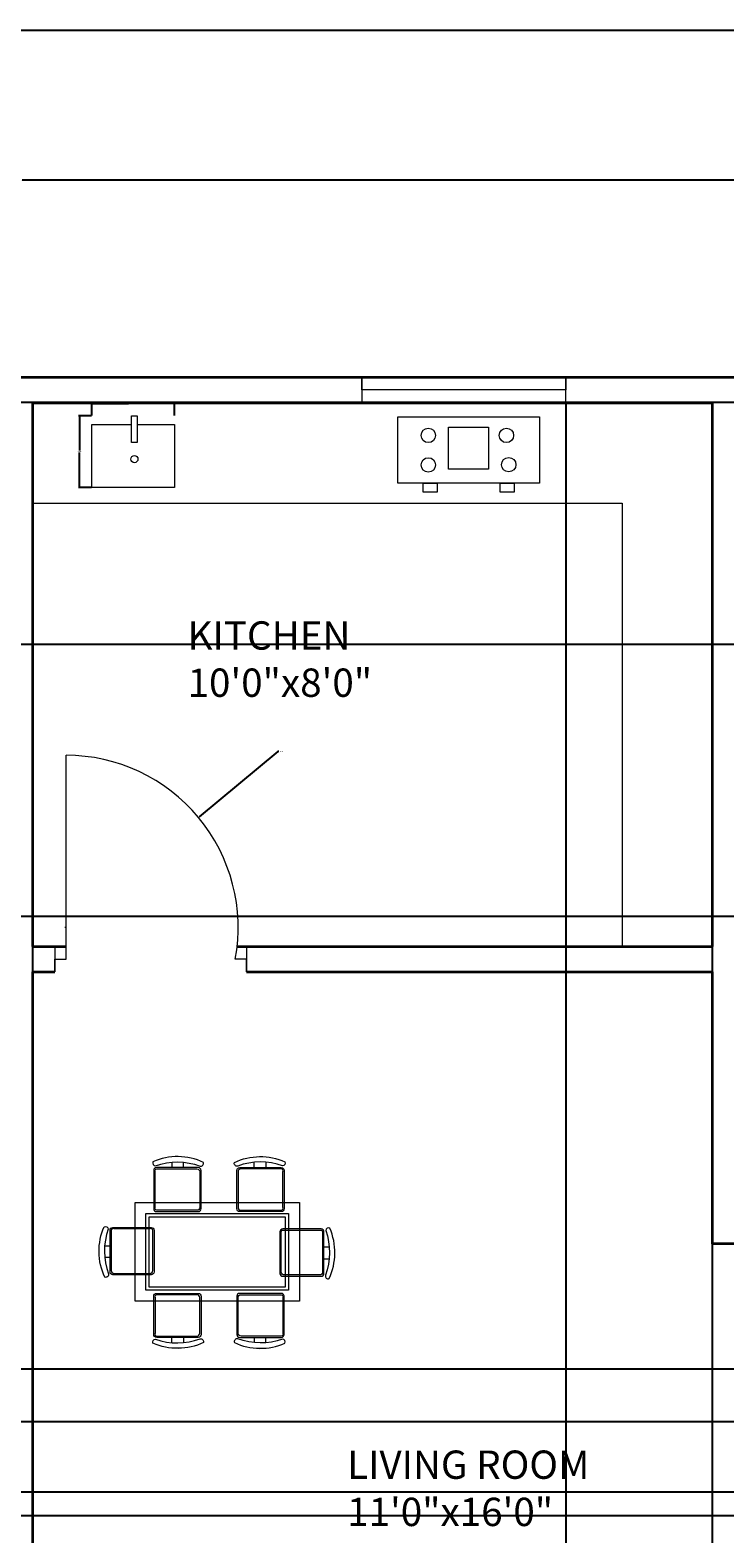
# Model space of a CAD drawing. Units: inches. Extents: x 1861 to 2564, y 1482 to 2317.
# Tile 10 of 11: x 2217 to 2339, y 2051 to 2317. Entities that reach past the tile are written whole.
import ezdxf

# ---------------------------------------------------------------- set-up
doc = ezdxf.new("R2010")
doc.units = ezdxf.units.IN
for name, color, linetype, lineweight in [('A-ANNO-DIMS', 2, 'Continuous', 18), ('A-ANNO-TTLB', 7, 'Continuous', 25), ('A-AREA-IDEN', 7, 'Continuous', 18), ('A-DOOR', 3, 'Continuous', 18), ('A-EQPM', 8, 'Continuous', 18), ('A-FLOR-CASE', 9, 'Continuous', 18), ('A-FLOR-FIXT', 8, 'Continuous', 18), ('A-FURN', 8, 'Continuous', 13), ('A-GLAZ', 4, 'Continuous', 18), ('A-WALL', 7, 'Continuous', 35)]:
    doc.layers.add(name, color=color, linetype=linetype, lineweight=lineweight)
doc.styles.get("Standard").update_dxf_attribs({"font": 'arial.ttf'})
doc.dimstyles.get("Standard").update_dxf_attribs({"dimtxt": 0.18, "dimasz": 0.18, "dimexe": 0.18, "dimexo": 0.0625, "dimgap": 0.09, "dimtad": 0, "dimtih": 1, "dimtoh": 1, "dimdec": 4, "dimzin": 0, "dimdsep": 46, "dimtxsty": 'Standard', "dimcen": 0.09, "dimadec": 0, "dimazin": 0, "dimtfac": 1, "dimtdec": 4, "dimtofl": 0, "dimtmove": 0, "dimatfit": 3, "dimfxl": 1, "dimtolj": 1, "dimtzin": 0, "dimarcsym": 0})

# ---------------------------------------------------------------- blocks, each defined once
blk = doc.blocks.new('SINK-KITCHEN')
blk.add_lwpolyline([(7.97, 11.14), (14.59, 11.14), (14.59, 0), (0, 0), (0, 11.14), (6.99, 11.14)])
blk.add_lwpolyline([(6.99, 12.66), (7.97, 12.66), (7.97, 7.92), (6.99, 7.92)], close=True)
blk.add_circle((7.5, 5.01), 0.628)
blk = doc.blocks.new('COOKTOP-4B')
for points in [[(-0.01, 13.28), (25.01, 13.28), (25.01, 1.58), (-0.01, 1.58)], [(8.91, 11.43), (16.01, 11.43), (16.01, 4.05), (8.91, 4.05)], [(4.47, 1.58), (6.95, 1.58), (6.95, 0), (4.47, 0)], [(18.04, 1.58), (20.51, 1.58), (20.51, 0), (18.04, 0)]]:
    blk.add_lwpolyline(points, close=True)
for centre in [(5.36, 10), (19.16, 10), (5.36, 4.79), (19.56, 4.83)]:
    blk.add_circle(centre, 1.27)
blk = doc.blocks.new('TABLE-DINING-RECT')
for points in [[(0, 17.4), (29.01, 17.4), (29.01, 0), (0, 0)], [(0, 17.4), (29.01, 17.4), (29.01, 0), (0, 0)], [(1.93, 15.47), (27.08, 15.47), (27.08, 1.93), (1.93, 1.93)], [(1.93, 15.47), (27.08, 15.47), (27.08, 1.93), (1.93, 1.93)], [(2.51, 14.89), (26.5, 14.89), (26.5, 2.51), (2.51, 2.51)], [(2.51, 14.89), (26.5, 14.89), (26.5, 2.51), (2.51, 2.51)]]:
    blk.add_lwpolyline(points, close=True)
blk = doc.blocks.new('*D22')
at = {"layer": 'A-ANNO-DIMS', "color": 0, "lineweight": -2, "transparency": 16777216}
for p, q in [((2227.72, 2248.64), (2227.72, 2250.94)), ((2227.9, 2250.76), (2234.16, 2250.76)), ((2242.13, 2250.76), (2235.87, 2250.76)), ((2242.31, 2248.64), (2242.31, 2250.94))]:
    blk.add_line(p, q, dxfattribs=at)
at = {"layer": 'A-ANNO-DIMS', "color": 0, "transparency": 16777216}
for points in [[(2227.9, 2250.79), (2227.9, 2250.73), (2227.72, 2250.76)], [(2242.13, 2250.79), (2242.13, 2250.73), (2242.31, 2250.76)]]:
    blk.add_solid(points, dxfattribs=at)
at = {"layer": 'Defpoints', "color": 0, "transparency": 16777216}
for p in [(2227.72, 2248.57), (2242.31, 2250.76), (2242.31, 2248.57)]:
    blk.add_point(p, dxfattribs=at)
at = {"layer": 'A-ANNO-DIMS', "color": 0, "transparency": 16777216, "insert": (2235.02, 2250.76), "char_height": 0.18, "attachment_point": 5}
blk.add_mtext('\\A1;SINK 15 TYP.', dxfattribs=at)
blk = doc.blocks.new('*D23')
at = {"layer": 'A-ANNO-DIMS', "color": 0, "lineweight": -2, "transparency": 16777216}
for p, q in [((2227.66, 2248.57), (2225.35, 2248.57)), ((2225.53, 2248.39), (2225.53, 2242.43)), ((2225.53, 2236.09), (2225.53, 2242.06)), ((2227.66, 2235.91), (2225.35, 2235.91))]:
    blk.add_line(p, q, dxfattribs=at)
at = {"layer": 'A-ANNO-DIMS', "color": 0, "transparency": 16777216}
for points in [[(2225.5, 2248.39), (2225.56, 2248.39), (2225.53, 2248.57)], [(2225.5, 2236.09), (2225.56, 2236.09), (2225.53, 2235.91)]]:
    blk.add_solid(points, dxfattribs=at)
at = {"layer": 'Defpoints', "color": 0, "transparency": 16777216}
for p in [(2225.53, 2248.57), (2227.72, 2248.57), (2227.72, 2235.91)]:
    blk.add_point(p, dxfattribs=at)
at = {"layer": 'A-ANNO-DIMS', "color": 0, "transparency": 16777216, "insert": (2225.53, 2242.24), "char_height": 0.18, "attachment_point": 5}
blk.add_mtext('\\A1;13 TYP.', dxfattribs=at)
blk = doc.blocks.new('*D34')
at = {"layer": 'A-ANNO-DIMS', "color": 0, "lineweight": -2, "transparency": 16777216}
for p, q in [((1927.74, 2255.45), (1927.74, 2290.37)), ((1927.92, 2290.19), (2214.59, 2290.19)), ((2502.06, 2290.19), (2215.38, 2290.19)), ((2502.24, 2255.45), (2502.24, 2290.37))]:
    blk.add_line(p, q, dxfattribs=at)
at = {"layer": 'A-ANNO-DIMS', "color": 0, "transparency": 16777216}
for points in [[(1927.92, 2290.22), (1927.92, 2290.16), (1927.74, 2290.19)], [(2502.06, 2290.22), (2502.06, 2290.16), (2502.24, 2290.19)]]:
    blk.add_solid(points, dxfattribs=at)
at = {"layer": 'Defpoints', "color": 0, "transparency": 16777216}
for p in [(2502.24, 2290.19), (1927.74, 2255.39), (2502.24, 2255.39)]:
    blk.add_point(p, dxfattribs=at)
at = {"layer": 'A-ANNO-DIMS', "color": 0, "transparency": 16777216, "insert": (2214.99, 2290.19), "char_height": 0.18, "attachment_point": 5}
blk.add_mtext('\\A1;574.5', dxfattribs=at)
blk = doc.blocks.new('*D37')
at = {"layer": 'A-ANNO-DIMS', "color": 0, "lineweight": -2, "transparency": 16777216}
for p, q in [((2311.38, 2250.82), (2311.38, 1545.6)), ((2337.24, 2250.82), (2337.24, 1545.6)), ((2311.56, 1545.78), (2323.91, 1545.78)), ((2337.06, 1545.78), (2324.7, 1545.78))]:
    blk.add_line(p, q, dxfattribs=at)
at = {"layer": 'A-ANNO-DIMS', "color": 0, "transparency": 16777216}
for points in [[(2311.56, 1545.81), (2311.56, 1545.75), (2311.38, 1545.78)], [(2337.06, 1545.81), (2337.06, 1545.75), (2337.24, 1545.78)]]:
    blk.add_solid(points, dxfattribs=at)
at = {"layer": 'Defpoints', "color": 0, "transparency": 16777216}
for p in [(2311.38, 2250.89), (2337.24, 2250.89), (2337.24, 1545.78)]:
    blk.add_point(p, dxfattribs=at)
at = {"layer": 'A-ANNO-DIMS', "color": 0, "transparency": 16777216, "insert": (2324.31, 1545.78), "char_height": 0.18, "attachment_point": 5}
blk.add_mtext('\\A1;25.86', dxfattribs=at)
blk = doc.blocks.new('*D60')
at = {"layer": 'A-ANNO-DIMS', "color": 0, "lineweight": -2, "transparency": 16777216}
for p, q in [((2497.68, 2208.17), (1892.76, 2208.17)), ((1892.94, 2207.99), (1892.94, 2184.35)), ((1892.94, 2160.35), (1892.94, 2183.99)), ((2497.68, 2160.17), (1892.76, 2160.17))]:
    blk.add_line(p, q, dxfattribs=at)
at = {"layer": 'A-ANNO-DIMS', "color": 0, "transparency": 16777216}
for points in [[(1892.91, 2207.99), (1892.97, 2207.99), (1892.94, 2208.17)], [(1892.91, 2160.35), (1892.97, 2160.35), (1892.94, 2160.17)]]:
    blk.add_solid(points, dxfattribs=at)
at = {"layer": 'Defpoints', "color": 0, "transparency": 16777216}
for p in [(1892.94, 2208.17), (2497.74, 2208.17), (2497.74, 2160.17)]:
    blk.add_point(p, dxfattribs=at)
at = {"layer": 'A-ANNO-DIMS', "color": 0, "transparency": 16777216, "insert": (1892.94, 2184.17), "char_height": 0.18, "attachment_point": 5}
blk.add_mtext('\\A1;48', dxfattribs=at)
blk = doc.blocks.new('*D61')
at = {"layer": 'A-ANNO-DIMS', "color": 0, "lineweight": -2, "transparency": 16777216}
for p, q in [((2008.8, 2080.33), (2537.22, 2080.33)), ((2537.04, 2080.15), (2537.04, 2069.66)), ((2537.04, 2058.82), (2537.04, 2069.3)), ((2008.8, 2058.64), (2537.22, 2058.64))]:
    blk.add_line(p, q, dxfattribs=at)
at = {"layer": 'A-ANNO-DIMS', "color": 0, "transparency": 16777216}
for points in [[(2537.01, 2080.15), (2537.07, 2080.15), (2537.04, 2080.33)], [(2537.01, 2058.82), (2537.07, 2058.82), (2537.04, 2058.64)]]:
    blk.add_solid(points, dxfattribs=at)
at = {"layer": 'Defpoints', "color": 0, "transparency": 16777216}
for p in [(2008.74, 2080.33), (2537.04, 2080.33), (2008.74, 2058.64)]:
    blk.add_point(p, dxfattribs=at)
at = {"layer": 'A-ANNO-DIMS', "color": 0, "transparency": 16777216, "insert": (2537.04, 2069.48), "char_height": 0.18, "attachment_point": 5}
blk.add_mtext('\\A1;21.693', dxfattribs=at)
blk = doc.blocks.new('*D63')
at = {"layer": 'A-ANNO-DIMS', "color": 0, "lineweight": -2, "transparency": 16777216}
for p, q in [((2497.68, 2250.89), (1892.76, 2250.89)), ((1892.94, 2250.71), (1892.94, 2229.71)), ((1892.94, 2208.35), (1892.94, 2229.35)), ((2497.68, 2208.17), (1892.76, 2208.17))]:
    blk.add_line(p, q, dxfattribs=at)
at = {"layer": 'A-ANNO-DIMS', "color": 0, "transparency": 16777216}
for points in [[(1892.91, 2250.71), (1892.97, 2250.71), (1892.94, 2250.89)], [(1892.91, 2208.35), (1892.97, 2208.35), (1892.94, 2208.17)]]:
    blk.add_solid(points, dxfattribs=at)
at = {"layer": 'Defpoints', "color": 0, "transparency": 16777216}
for p in [(2497.74, 2250.89), (1892.94, 2208.17), (2497.74, 2208.17)]:
    blk.add_point(p, dxfattribs=at)
at = {"layer": 'A-ANNO-DIMS', "color": 0, "transparency": 16777216, "insert": (1892.94, 2229.53), "char_height": 0.18, "attachment_point": 5}
blk.add_mtext('\\A1;42.71', dxfattribs=at)
blk = doc.blocks.new('*D64')
at = {"layer": 'A-ANNO-DIMS', "color": 0, "lineweight": -2, "transparency": 16777216}
for p, q in [((2497.68, 2070.96), (1892.76, 2070.96)), ((1892.94, 2070.78), (1892.94, 2062.85)), ((1892.94, 2054.57), (1892.94, 2062.49)), ((2497.68, 2054.39), (1892.76, 2054.39))]:
    blk.add_line(p, q, dxfattribs=at)
at = {"layer": 'A-ANNO-DIMS', "color": 0, "transparency": 16777216}
for points in [[(1892.91, 2070.78), (1892.97, 2070.78), (1892.94, 2070.96)], [(1892.91, 2054.57), (1892.97, 2054.57), (1892.94, 2054.39)]]:
    blk.add_solid(points, dxfattribs=at)
at = {"layer": 'Defpoints', "color": 0, "transparency": 16777216}
for p in [(2497.74, 2070.96), (1892.94, 2054.39), (2497.74, 2054.39)]:
    blk.add_point(p, dxfattribs=at)
at = {"layer": 'A-ANNO-DIMS', "color": 0, "transparency": 16777216, "insert": (1892.94, 2062.67), "char_height": 0.18, "attachment_point": 5}
blk.add_mtext('\\A1;16.57', dxfattribs=at)
blk = doc.blocks.new('*D71')
at = {"layer": 'A-ANNO-DIMS', "color": 0, "lineweight": -2, "transparency": 16777216}
for p, q in [((2212.74, 2250.82), (2212.74, 1545.6)), ((2217.24, 2250.82), (2217.24, 1545.6)), ((2212.92, 1545.78), (2214.73, 1545.78)), ((2217.06, 1545.78), (2215.25, 1545.78))]:
    blk.add_line(p, q, dxfattribs=at)
at = {"layer": 'A-ANNO-DIMS', "color": 0, "transparency": 16777216}
for points in [[(2212.92, 1545.81), (2212.92, 1545.75), (2212.74, 1545.78)], [(2217.06, 1545.81), (2217.06, 1545.75), (2217.24, 1545.78)]]:
    blk.add_solid(points, dxfattribs=at)
at = {"layer": 'Defpoints', "color": 0, "transparency": 16777216}
for p in [(2212.74, 2250.89), (2217.24, 2250.89), (2217.24, 1545.78)]:
    blk.add_point(p, dxfattribs=at)
at = {"layer": 'A-ANNO-DIMS', "color": 0, "transparency": 16777216, "insert": (2214.99, 1545.78), "char_height": 0.18, "attachment_point": 5}
blk.add_mtext('\\A1;4.5', dxfattribs=at)
blk = doc.blocks.new('*D77')
at = {"layer": 'A-ANNO-DIMS', "color": 0, "lineweight": -2, "transparency": 16777216}
for p, q in [((2260.57, 2189.3), (2246.67, 2177.77)), ((2260.75, 2189.3), (2260.57, 2189.3)), ((2223.14, 2158.15), (2223.14, 2158.33)), ((2223.05, 2158.24), (2223.23, 2158.24))]:
    blk.add_line(p, q, dxfattribs=at)
at = {"layer": 'A-ANNO-DIMS', "color": 0, "transparency": 16777216}
blk.add_solid([(2246.65, 2177.79), (2246.69, 2177.74), (2246.53, 2177.65)], dxfattribs=at)
at = {"layer": 'Defpoints', "color": 0, "transparency": 16777216}
for p in [(2246.53, 2177.65), (2223.14, 2158.24)]:
    blk.add_point(p, dxfattribs=at)
at = {"layer": 'A-ANNO-DIMS', "color": 0, "transparency": 16777216, "insert": (2261.16, 2189.3), "char_height": 0.18, "attachment_point": 5}
blk.add_mtext('\\A1;R30.4', dxfattribs=at)

msp = doc.modelspace()

# ---------------------------------------------------------------- linework, layer by layer
at = {"layer": 'A-ANNO-TTLB'}
msp.add_lwpolyline([(1861.1332, 2316.6589), (2563.8077, 2316.6589), (2563.8077, 1482.0728), (1861.1332, 1482.0728)], close=True, dxfattribs=at)
at = {"layer": 'A-DOOR'}
for p, q in [((2223.1437, 2152.6354), (2223.1437, 2188.6354)), ((2221.1437, 2154.8854), (2221.1437, 2150.3854)), ((2255.02, 2154.8854), (2255.02, 2150.3854)), ((2221.1437, 2150.3854), (2221.1437, 2152.6354)), ((2221.1437, 2152.6354), (2223.1437, 2152.6354)), ((2255.02, 2152.6354), (2253.02, 2152.6354)), ((2255.02, 2150.3854), (2255.02, 2152.6354))]:
    msp.add_line(p, q, dxfattribs=at)
msp.add_arc((2223.1437, 2158.2382), 30.3972, 349.378469, 90, dxfattribs=at)
at = {"layer": 'A-FLOR-CASE'}
for p, q in [((2217.2393, 2233.1335), (2321.3686, 2233.1335)), ((2321.3686, 2233.1335), (2321.3686, 2154.8854))]:
    msp.add_line(p, q, dxfattribs=at)
at = {"layer": 'A-FURN'}
for points in [[(2238.9215, 2116.179, -0.17580919), (2246.8232, 2116.1192, 0.57839206), (2247.4218, 2116.7774, 0.21452438), (2238.5025, 2116.8971, 0.55201397), (2238.9215, 2116.179, -0.06507904)], [(2238.9215, 2116.1787, -0.17580919), (2246.8232, 2116.1189, 0.57839206), (2247.4218, 2116.7771, 0.21452438), (2238.5025, 2116.8968, 0.55201397), (2238.9215, 2116.1787, -0.06507904)], [(2246.488, 2115.8619), (2239.1523, 2115.8619, 0.41421356), (2238.6391, 2115.3487), (2238.6391, 2108.6036, 0.41421356), (2239.1523, 2108.0904), (2246.488, 2108.0904, 0.41421356), (2247.0012, 2108.6036), (2247.0012, 2115.3487, 0.41421356), (2246.488, 2115.8619)], [(2246.488, 2115.8616), (2239.1523, 2115.8616, 0.41421356), (2238.6391, 2115.3484), (2238.6391, 2108.6033, 0.41421356), (2239.1523, 2108.0901), (2246.488, 2108.0901, 0.41421356), (2247.0012, 2108.6033), (2247.0012, 2115.3484, 0.41421356), (2246.488, 2115.8616)], [(2243.9113, 2115.8619), (2243.9113, 2116.7896, -0.06475861)], [(2243.9113, 2115.8616), (2243.9113, 2116.7893, -0.06475861)], [(2253.4754, 2116.1192, -0.57839206), (2252.8768, 2116.7774, -0.21452438), (2261.7962, 2116.8971, -0.55201397), (2261.3771, 2116.179, 0.1758092), (2253.4754, 2116.1192)], [(2253.4754, 2116.1189, -0.57839206), (2252.8768, 2116.7771, -0.21452438), (2261.7962, 2116.8968, -0.55201397), (2261.3771, 2116.1787, 0.1758092), (2253.4754, 2116.1189)], [(2261.1463, 2115.8619, -0.41421356), (2261.6595, 2115.3487), (2261.6595, 2108.6036, -0.41421356), (2261.1463, 2108.0904), (2253.8107, 2108.0904, -0.41421356), (2253.2974, 2108.6036), (2253.2974, 2115.3487, -0.41421356), (2253.8107, 2115.8619), (2261.1463, 2115.8619)], [(2261.1463, 2115.8616, -0.41421356), (2261.6596, 2115.3484), (2261.6596, 2108.6033, -0.41421356), (2261.1463, 2108.0901), (2253.8107, 2108.0901, -0.41421356), (2253.2975, 2108.6033), (2253.2975, 2115.3484, -0.41421356), (2253.8107, 2115.8616), (2261.1463, 2115.8616)], [(2256.3873, 2115.8619), (2256.3873, 2116.7896, 0.06475861)], [(2256.3873, 2115.8616), (2256.3873, 2116.7893, 0.06475861)], [(2230.6548, 2097.0976, -0.57839206), (2229.9966, 2096.499, -0.21452438), (2229.8769, 2105.4183, -0.55201397), (2230.595, 2104.9993, 0.17580937), (2230.6548, 2097.0976)], [(2230.6548, 2097.0973, -0.57839206), (2229.9966, 2096.4987, -0.21452438), (2229.8769, 2105.418, -0.55201397), (2230.595, 2104.999, 0.17580937), (2230.6548, 2097.0973)], [(2230.9121, 2104.7685, -0.41421356), (2231.4253, 2105.2817), (2238.1703, 2105.2817, -0.41421356), (2238.6835, 2104.7685), (2238.6835, 2097.4328, -0.41421356), (2238.1703, 2096.9196), (2231.4253, 2096.9196, -0.41421356), (2230.9121, 2097.4328), (2230.9121, 2104.7685)], [(2230.9121, 2104.7682, -0.41421356), (2231.4253, 2105.2814), (2238.1703, 2105.2814, -0.41421356), (2238.6836, 2104.7682), (2238.6836, 2097.4325, -0.41421356), (2238.1703, 2096.9193), (2231.4253, 2096.9193, -0.41421356), (2230.9121, 2097.4325), (2230.9121, 2104.7682)], [(2269.0045, 2104.7481, -0.17580919), (2268.9447, 2096.8464, 0.57839206), (2269.6029, 2096.2478, 0.21452438), (2269.7226, 2105.1671, 0.55201397), (2269.0045, 2104.7481, -0.06507904)], [(2269.0045, 2104.7478, -0.17580919), (2268.9447, 2096.8461, 0.57839206), (2269.6029, 2096.2474, 0.21452438), (2269.7226, 2105.1668, 0.55201397), (2269.0045, 2104.7478, -0.06507904)], [(2268.6874, 2104.5173, 0.41421356), (2268.1742, 2105.0305), (2261.4292, 2105.0305, 0.41421356), (2260.916, 2104.5173), (2260.916, 2097.1816, 0.41421356), (2261.4292, 2096.6684), (2268.1742, 2096.6684, 0.41421356), (2268.6874, 2097.1816), (2268.6874, 2104.5173)], [(2268.6874, 2104.517, 0.41421356), (2268.1742, 2105.0302), (2261.4292, 2105.0302, 0.41421356), (2260.916, 2104.517), (2260.916, 2097.1813, 0.41421356), (2261.4292, 2096.6681), (2268.1742, 2096.6681, 0.41421356), (2268.6874, 2097.1813), (2268.6874, 2104.517)], [(2230.9121, 2100.0095), (2229.9844, 2100.0095, 0.06475861)], [(2230.9121, 2100.0092), (2229.9844, 2100.0092, 0.06475861)], [(2268.6874, 2099.7583), (2269.6151, 2099.7583, -0.06475861)], [(2268.6874, 2099.758), (2269.6151, 2099.758, -0.06475861)], [(2246.488, 2085.8786), (2239.1523, 2085.8786, -0.41421356), (2238.6391, 2086.3919), (2238.6391, 2093.1369, -0.41421356), (2239.1523, 2093.6501), (2246.488, 2093.6501, -0.41421356), (2247.0012, 2093.1369), (2247.0012, 2086.3919, -0.41421356), (2246.488, 2085.8786)], [(2246.488, 2085.8783), (2239.1523, 2085.8783, -0.41421356), (2238.6391, 2086.3916), (2238.6391, 2093.1366, -0.41421356), (2239.1523, 2093.6498), (2246.488, 2093.6498, -0.41421356), (2247.0012, 2093.1366), (2247.0012, 2086.3916, -0.41421356), (2246.488, 2085.8783)], [(2261.1463, 2085.8786, 0.41421356), (2261.6595, 2086.3919), (2261.6595, 2093.1369, 0.41421356), (2261.1463, 2093.6501), (2253.8107, 2093.6501, 0.41421356), (2253.2974, 2093.1369), (2253.2974, 2086.3919, 0.41421356), (2253.8107, 2085.8786), (2261.1463, 2085.8786)], [(2261.1463, 2085.8783, 0.41421356), (2261.6596, 2086.3916), (2261.6596, 2093.1366, 0.41421356), (2261.1463, 2093.6498), (2253.8107, 2093.6498, 0.41421356), (2253.2975, 2093.1366), (2253.2975, 2086.3916, 0.41421356), (2253.8107, 2085.8783), (2261.1463, 2085.8783)], [(2246.8232, 2085.6213, -0.57839206), (2247.4218, 2084.9631, -0.21452438), (2238.5025, 2084.8434, -0.55201397), (2238.9215, 2085.5615, 0.17580929), (2246.8232, 2085.6213)], [(2246.8232, 2085.621, -0.57839206), (2247.4218, 2084.9628, -0.21452438), (2238.5025, 2084.8431, -0.55201397), (2238.9215, 2085.5612, 0.17580929), (2246.8232, 2085.621)], [(2243.9113, 2085.8786), (2243.9113, 2084.9509, 0.06475861)], [(2243.9113, 2085.8783), (2243.9113, 2084.9506, 0.06475861)], [(2261.3771, 2085.5615, -0.17580928), (2253.4754, 2085.6213, 0.57839206), (2252.8768, 2084.9631, 0.21452438), (2261.7962, 2084.8434, 0.55201397), (2261.3771, 2085.5615, -0.06507904)], [(2261.3771, 2085.5612, -0.17580928), (2253.4754, 2085.621, 0.57839206), (2252.8768, 2084.9628, 0.21452438), (2261.7962, 2084.8431, 0.55201397), (2261.3771, 2085.5612, -0.06507904)], [(2256.3873, 2085.8786), (2256.3873, 2084.9509, -0.06475861)], [(2256.3873, 2085.8783), (2256.3873, 2084.9506, -0.06475861)]]:
    msp.add_lwpolyline(points, format="xyb", dxfattribs=at)
for points in [[(2241.858, 2116.8065), (2241.858, 2115.8619)], [(2241.858, 2116.8062), (2241.858, 2115.8616)], [(2258.4407, 2116.8065), (2258.4407, 2115.8619)], [(2258.4407, 2116.8062), (2258.4407, 2115.8616)], [(2229.9675, 2102.0629), (2230.9121, 2102.0629)], [(2229.9675, 2102.0625), (2230.9121, 2102.0625)], [(2269.632, 2101.8116), (2268.6874, 2101.8116)], [(2269.632, 2101.8113), (2268.6874, 2101.8113)], [(2241.858, 2084.9341), (2241.858, 2085.8786)], [(2241.858, 2084.9337), (2241.858, 2085.8783)], [(2258.4407, 2084.9341), (2258.4407, 2085.8786)], [(2258.4407, 2084.9337), (2258.4407, 2085.8783)]]:
    msp.add_lwpolyline(points, dxfattribs=at)
for points in [[(2239.1554, 2115.6307), (2246.2568, 2115.6307, -0.41421356), (2246.77, 2115.1175), (2246.77, 2108.8349, -0.41421356), (2246.2568, 2108.3216), (2239.1554, 2108.3216, -0.51206948), (2238.8703, 2108.8349), (2238.8703, 2115.1175, -0.51206948)], [(2239.1554, 2115.6304), (2246.2568, 2115.6304, -0.41421356), (2246.77, 2115.1171), (2246.77, 2108.8345, -0.41421356), (2246.2568, 2108.3213), (2239.1554, 2108.3213, -0.51206948), (2238.8703, 2108.8345), (2238.8703, 2115.1171, -0.51206948)], [(2261.1432, 2115.6307), (2254.0419, 2115.6307, 0.41421356), (2253.5287, 2115.1175), (2253.5287, 2108.8349, 0.41421356), (2254.0419, 2108.3216), (2261.1432, 2108.3216, 0.51206948), (2261.4283, 2108.8349), (2261.4283, 2115.1175, 0.51206948)], [(2261.1432, 2115.6304), (2254.0419, 2115.6304, 0.41421356), (2253.5287, 2115.1171), (2253.5287, 2108.8345, 0.41421356), (2254.0419, 2108.3213), (2261.1432, 2108.3213, 0.51206948), (2261.4284, 2108.8345), (2261.4284, 2115.1171, 0.51206948)], [(2231.1433, 2104.7654), (2231.1433, 2097.664, 0.41421356), (2231.6565, 2097.1508), (2237.9391, 2097.1508, 0.41421356), (2238.4523, 2097.664), (2238.4523, 2104.7654, 0.51206948), (2237.9391, 2105.0505), (2231.6565, 2105.0505, 0.51206948)], [(2231.1433, 2104.7651), (2231.1433, 2097.6637, 0.41421356), (2231.6565, 2097.1505), (2237.9391, 2097.1505, 0.41421356), (2238.4524, 2097.6637), (2238.4524, 2104.7651, 0.51206948), (2237.9391, 2105.0502), (2231.6565, 2105.0502, 0.51206948)], [(2268.4562, 2104.5142), (2268.4562, 2097.4128, -0.41421356), (2267.943, 2096.8996), (2261.6604, 2096.8996, -0.41421356), (2261.1472, 2097.4128), (2261.1472, 2104.5142, -0.51206948), (2261.6604, 2104.7993), (2267.943, 2104.7993, -0.51206948)], [(2268.4562, 2104.5139), (2268.4562, 2097.4125, -0.41421356), (2267.943, 2096.8993), (2261.6604, 2096.8993, -0.41421356), (2261.1472, 2097.4125), (2261.1472, 2104.5139, -0.51206948), (2261.6604, 2104.799), (2267.943, 2104.799, -0.51206948)], [(2239.1554, 2086.1099), (2246.2568, 2086.1099, 0.41421356), (2246.77, 2086.6231), (2246.77, 2092.9057, 0.41421356), (2246.2568, 2093.4189), (2239.1554, 2093.4189, 0.51206948), (2238.8703, 2092.9057), (2238.8703, 2086.6231, 0.51206948)], [(2239.1554, 2086.1095), (2246.2568, 2086.1095, 0.41421356), (2246.77, 2086.6228), (2246.77, 2092.9054, 0.41421356), (2246.2568, 2093.4186), (2239.1554, 2093.4186, 0.51206948), (2238.8703, 2092.9054), (2238.8703, 2086.6228, 0.51206948)], [(2261.1432, 2086.1099), (2254.0419, 2086.1099, -0.41421356), (2253.5287, 2086.6231), (2253.5287, 2092.9057, -0.41421356), (2254.0419, 2093.4189), (2261.1432, 2093.4189, -0.51206948), (2261.4283, 2092.9057), (2261.4283, 2086.6231, -0.51206948)], [(2261.1432, 2086.1095), (2254.0419, 2086.1095, -0.41421356), (2253.5287, 2086.6228), (2253.5287, 2092.9054, -0.41421356), (2254.0419, 2093.4186), (2261.1432, 2093.4186, -0.51206948), (2261.4284, 2092.9054), (2261.4284, 2086.6228, -0.51206948)]]:
    msp.add_lwpolyline(points, format="xyb", close=True, dxfattribs=at)
at = {"layer": 'A-GLAZ'}
for p, q in [((2275.3789, 2253.1354), (2275.3789, 2255.3854)), ((2275.3789, 2255.3854), (2275.3789, 2250.8854)), ((2311.3789, 2250.8854), (2311.3789, 2255.3854)), ((2311.3789, 2255.3854), (2311.3789, 2253.1354)), ((2311.3789, 2253.1354), (2275.3789, 2253.1354))]:
    msp.add_line(p, q, dxfattribs=at)
at = {"layer": 'A-WALL'}
for p, q in [((1927.7393, 2255.3854), (2502.2393, 2255.3854)), ((2217.2393, 2250.8854), (2217.2393, 2154.8854)), ((2217.2393, 2250.8854), (2337.2393, 2250.8854)), ((2337.2393, 2250.8854), (2337.2393, 2154.8854)), ((2217.2393, 2154.8854), (2223.1437, 2154.8854)), ((2253.3554, 2154.8854), (2337.2393, 2154.8854)), ((2217.2393, 2150.3854), (2217.2393, 1863.6796)), ((2217.2393, 2150.3854), (2221.1437, 2150.3854)), ((2255.02, 2150.3854), (2337.2393, 2150.3854)), ((2337.2393, 2150.3854), (2337.2393, 2102.3854)), ((2341.7393, 2102.3854), (2337.2393, 2102.3854))]:
    msp.add_line(p, q, dxfattribs=at)

# ---------------------------------------------------------------- block references
at = {"layer": 'A-EQPM'}
msp.add_blockref('COOKTOP-4B', (2281.753, 2235.1063), dxfattribs=at)
at = {"layer": 'A-FLOR-FIXT'}
msp.add_blockref('SINK-KITCHEN', (2227.7181, 2235.91), dxfattribs=at)
at = {"layer": 'A-FURN'}
msp.add_blockref('TABLE-DINING-RECT', (2235.3338, 2092.2627), dxfattribs=at)

# ---------------------------------------------------------------- texts
at = {"layer": 'A-AREA-IDEN', "char_height": 5, "attachment_point": 1}
for s, width, insert in [('KITCHEN\\P10\'0"x8\'0"', 82.755468, (2244.6079, 2212.2885)), ('LIVING ROOM\\P11\'0"x16\'0"', 138.970895, (2272.7816, 2065.9065))]:
    msp.add_mtext_dynamic_manual_height_columns(s, width=width, gutter_width=12.5, heights=[0], dxfattribs=dict(at, insert=insert))

# ---------------------------------------------------------------- dimensions: what is measured, and where the dimension line sits
at = {"layer": 'A-ANNO-DIMS'}
for base, p1, p2, override, picture, middle in [((2502.2393, 2290.1854), (1927.7393, 2255.3854), (2502.2393, 2255.3854), {"dimdec": 1, "dimlfac": 1, "dimrnd": 0, "dimzin": 0, "dimdsep": 46, "dimlunit": 2}, '*D34', (2214.9893, 2290.1854)), ((2217.2393, 1545.7777), (2212.7393, 2250.8854), (2217.2393, 2250.8854), {"dimdec": 1, "dimlfac": 1, "dimrnd": 0, "dimzin": 0, "dimdsep": 46, "dimlunit": 2}, '*D71', (2214.9893, 1545.7777)), ((2337.2393, 1545.7777), (2311.3789, 2250.8854), (2337.2393, 2250.8854), {"dimdec": 2, "dimlfac": 1, "dimrnd": 0, "dimzin": 0, "dimdsep": 46, "dimlunit": 2}, '*D37', (2324.3091, 1545.7777))]:
    dim = msp.add_linear_dim(base=base, p1=p1, p2=p2, dimstyle='Standard', override=override, dxfattribs=at)
    dim.commit()
    dim.dimension.update_dxf_attribs({"geometry": picture, "text_midpoint": middle})
for base, p1, p2, override, picture, middle in [((1892.9393, 2208.1728), (2497.7393, 2250.8854), (2497.7393, 2208.1728), {"dimdec": 2, "dimlfac": 1, "dimrnd": 0, "dimzin": 0, "dimdsep": 46, "dimlunit": 2}, '*D63', (1892.9393, 2229.5291)), ((1892.9393, 2208.1728), (2497.7393, 2160.1728), (2497.7393, 2208.1728), {"dimdec": 0, "dimlfac": 1, "dimrnd": 0, "dimzin": 0, "dimdsep": 46, "dimlunit": 2}, '*D60', (1892.9393, 2184.1728)), ((2537.0393, 2080.3283), (2008.7393, 2058.6356), (2008.7393, 2080.3283), {"dimdec": 3, "dimlfac": 1, "dimrnd": 0, "dimzin": 0, "dimdsep": 46, "dimlunit": 2}, '*D61', (2537.0393, 2069.4819)), ((1892.9393, 2054.3854), (2497.7393, 2070.957), (2497.7393, 2054.3854), {"dimdec": 2, "dimlfac": 1, "dimrnd": 0, "dimzin": 0, "dimdsep": 46, "dimlunit": 2}, '*D64', (1892.9393, 2062.6712))]:
    dim = msp.add_linear_dim(base=base, p1=p1, p2=p2, angle=90, dimstyle='Standard', override=override, dxfattribs=at)
    dim.commit()
    dim.dimension.update_dxf_attribs({"geometry": picture, "text_midpoint": middle})
dim = msp.add_linear_dim(base=(2225.532, 2248.5739), p1=(2227.7208, 2235.9122), p2=(2227.7208, 2248.5739), angle=90, text='<> TYP.', dimstyle='Standard', override={"dimdec": 0, "dimlfac": 1, "dimrnd": 0, "dimzin": 0, "dimdsep": 46, "dimlunit": 2}, dxfattribs=at)
dim.commit()
dim.dimension.update_dxf_attribs({"geometry": '*D23', "text_midpoint": (2225.532, 2242.2431)})
dim = msp.add_linear_dim(base=(2242.3126, 2250.7627), p1=(2227.7208, 2248.5739), p2=(2242.3126, 2248.5739), text='SINK <> TYP.', dimstyle='Standard', override={"dimdec": 0, "dimlfac": 1, "dimrnd": 0, "dimzin": 0, "dimdsep": 46, "dimlunit": 2}, dxfattribs=at)
dim.commit()
dim.dimension.update_dxf_attribs({"geometry": '*D22', "text_midpoint": (2235.0167, 2250.7627)})
dim = msp.add_radius_dim(center=(2223.1437, 2158.2382), mpoint=(2246.5347, 2177.6508), dimstyle='Standard', override={"dimdec": 1, "dimlfac": 1, "dimrnd": 0, "dimzin": 0, "dimdsep": 46, "dimlunit": 2}, dxfattribs=at)
dim.commit()
dim.dimension.update_dxf_attribs({"geometry": '*D77', "text_midpoint": (2261.1589, 2189.2983), "dimtype": 164})

doc.saveas('drawing.dxf')
